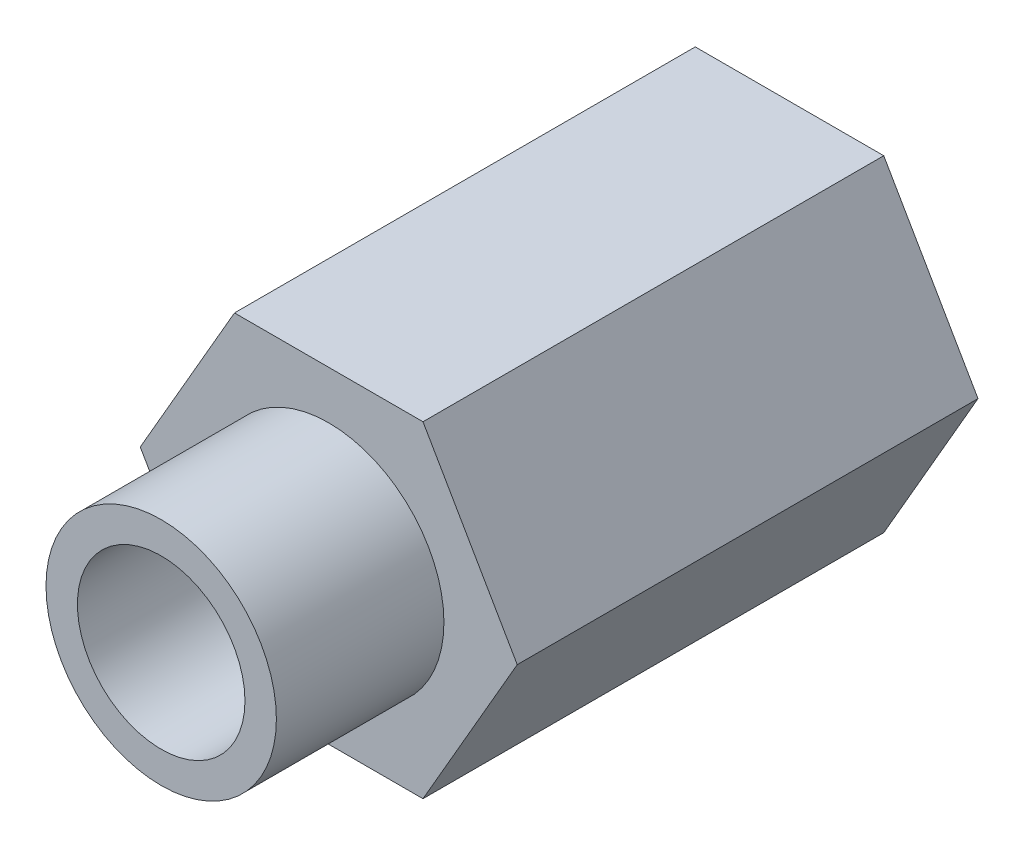
from build123d import *

# Parameters (mm, degrees)
HEX_BODY_22MM_DEPTH       = 22
SPIGOT_SKETCH_11_R        = 5.5
SPIGOT_11X8_DEPTH         = 8
SPIGOT_BORE_SKETCH_R      = 4
SPIGOT_THROUGH_BORE_DEPTH = 33.276152187
HEX_BORE_SKETCH_12_R      = 6
HEX_BORE_12X15_DEPTH      = 15


with BuildPart() as part:
    # Hex Profile Sketch → Hex Body 22mm (new body)
    with BuildSketch(Plane.XY):
        Polygon((9, 0), (4.5, 7.794228634), (-4.5, 7.794228634), (-9, 0), (-4.5, -7.794228634), (4.5, -7.794228634), align=None)
    extrude(amount=HEX_BODY_22MM_DEPTH)

    # Spigot Sketch Ø11 → Spigot Ø11x8 (add)
    with BuildSketch(Plane.XY.offset(22)):
        Circle(SPIGOT_SKETCH_11_R)
    extrude(amount=SPIGOT_11X8_DEPTH)

    # Spigot Bore Sketch → Spigot Through Bore (cut, through all)
    with BuildSketch(Plane.XY.offset(30)):
        Circle(SPIGOT_BORE_SKETCH_R)
    extrude(amount=-SPIGOT_THROUGH_BORE_DEPTH, mode=Mode.SUBTRACT)

    # Hex Bore Sketch Ø12 → Hex Bore Ø12x15 (cut)
    with BuildSketch(Plane(origin=(0, 0, 0), x_dir=(-1, 0, 0), z_dir=(0, 0, -1))):
        Circle(HEX_BORE_SKETCH_12_R)
    extrude(amount=-HEX_BORE_12X15_DEPTH, mode=Mode.SUBTRACT)


solid = part.part
